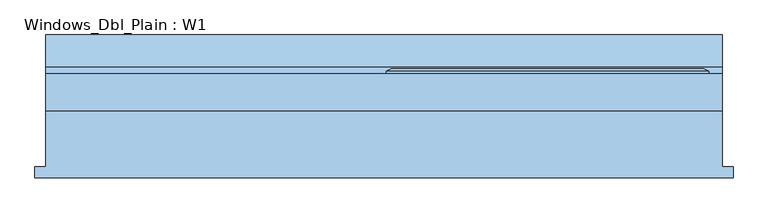
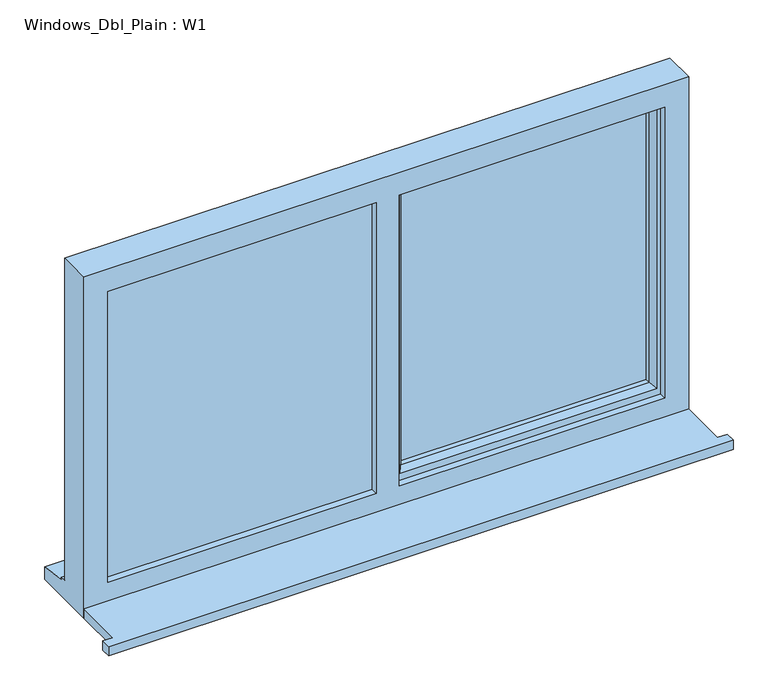
"""IFC4 building model written with IfcOpenShell, lengths in millimetres: window geometry, Windows_Dbl_Plain : W1."""

from ifc_helpers import new_model, si_unit, frame, origin, place, context, project, spatial, polyline, outline, extrude, faceted_brep, source, transform, mapped, element, save


def windows_dbl_plain_w1_b9c38b89(model_context):
    return source(origin(), model_context, "Body", "SolidModel", [
        extrude(outline(polyline([(-1072.0, -146.0834322), (-1072.0, -121.0834322), (-1047.0, -121.0834322), (-1047.0, 4.9965678), (477.0, 4.9965678), (477.0, -121.0834322), (502.0, -121.0834322), (502.0, -146.0834322), (-1072.0, -146.0834322)])), frame((0.0, 0.0, 1200.0), z_axis=(0.0, 0.0, 1.0), x_axis=(1.0, 0.0, 0.0)), (0.0, 0.0, 1.0), 25.0),
        faceted_brep([(-280.0, 87.9965678, 2080.0), (-280.0, 93.7700705, 2080.0), (-280.0, 93.7700705, 1253.0), (-280.0, 87.9965678, 1253.0), (-270.0, 22.9965678, 2070.0), (-270.0, 87.9965678, 2070.0), (-270.0, 87.9965678, 1263.0), (-270.0, 22.9965678, 1263.0), (-230.0, 37.4894677, 2030.0), (-240.1480377, 22.9965678, 2040.1480377), (-240.1480377, 22.9965678, 1292.8519623), (-230.0, 37.4894677, 1303.0), (-230.0, 51.9965678, 2030.0), (-230.0, 51.9965678, 1303.0), (-240.0, 75.9965678, 2040.0), (-240.0, 51.9965678, 2040.0), (-240.0, 51.9965678, 1293.0), (-240.0, 75.9965678, 1293.0), (-230.0, 93.7700705, 2030.0), (-230.0, 75.9965678, 2030.0), (-230.0, 75.9965678, 1303.0), (-230.0, 93.7700705, 1303.0), (-247.4457548, 99.5435732, 2047.4457548), (-247.4457548, 99.5435732, 1285.5542452), (-269.2153903, 99.5435732, 2069.2153903), (-269.2153903, 99.5435732, 1263.7846097), (447.0, 93.7700705, 1253.0), (447.0, 87.9965678, 1253.0), (437.0, 87.9965678, 1263.0), (437.0, 22.9965678, 1263.0), (407.1480377, 22.9965678, 1292.8519623), (397.0, 37.4894677, 1303.0), (397.0, 51.9965678, 1303.0), (407.0, 51.9965678, 1293.0), (407.0, 75.9965678, 1293.0), (397.0, 75.9965678, 1303.0), (397.0, 93.7700705, 1303.0), (414.4457548, 99.5435732, 1285.5542452), (436.2153903, 99.5435732, 1263.7846097), (447.0, 93.7700705, 2080.0), (447.0, 87.9965678, 2080.0), (437.0, 87.9965678, 2070.0), (437.0, 22.9965678, 2070.0), (407.1480377, 22.9965678, 2040.1480377), (397.0, 37.4894677, 2030.0), (397.0, 51.9965678, 2030.0), (407.0, 51.9965678, 2040.0), (407.0, 75.9965678, 2040.0), (397.0, 75.9965678, 2030.0), (397.0, 93.7700705, 2030.0), (414.4457548, 99.5435732, 2047.4457548), (436.2153903, 99.5435732, 2069.2153903)], [[[0, 1, 2, 3]], [[4, 5, 6, 7]], [[8, 9, 10, 11]], [[12, 8, 11, 13]], [[14, 15, 16, 17]], [[18, 19, 20, 21]], [[22, 18, 21, 23]], [[1, 24, 25, 2]], [[3, 2, 26, 27]], [[7, 6, 28, 29]], [[11, 10, 30, 31]], [[13, 11, 31, 32]], [[17, 16, 33, 34]], [[21, 20, 35, 36]], [[23, 21, 36, 37]], [[2, 25, 38, 26]], [[27, 26, 39, 40]], [[29, 28, 41, 42]], [[31, 30, 43, 44]], [[32, 31, 44, 45]], [[34, 33, 46, 47]], [[36, 35, 48, 49]], [[37, 36, 49, 50]], [[26, 38, 51, 39]], [[40, 39, 1, 0]], [[3, 27, 40, 0], [5, 41, 28, 6]], [[42, 41, 5, 4]], [[7, 29, 42, 4], [9, 43, 30, 10]], [[44, 43, 9, 8]], [[45, 44, 8, 12]], [[15, 46, 33, 16], [13, 32, 45, 12]], [[47, 46, 15, 14]], [[17, 34, 47, 14], [19, 48, 35, 20]], [[49, 48, 19, 18]], [[50, 49, 18, 22]], [[24, 51, 38, 25], [23, 37, 50, 22]], [[39, 51, 24, 1]]]),
        extrude(outline(polyline([(2050.0, -310.0), (2070.0, -310.0), (2070.0, -1007.0), (1263.0, -1007.0), (1263.0, -310.0), (1283.0, -310.0), (1283.0, -987.0), (2050.0, -987.0), (2050.0, -310.0)])), frame((0.0, 46.9965678, 0.0), z_axis=(0.0, 1.0, 0.0), x_axis=(0.0, 0.0, 1.0)), (0.0, 0.0, 1.0), 41.0),
        faceted_brep([(477.0, 4.9965678, 2110.0), (-1047.0, 4.9965678, 2110.0), (-1047.0, 4.9965678, 1200.0), (477.0, 4.9965678, 1200.0), (417.0, 4.9965678, 2050.0), (417.0, 4.9965678, 1275.0), (-252.0, 4.9965678, 1275.0), (-252.0, 4.9965678, 2050.0), (-310.0, 4.9965678, 2050.0), (-310.0, 4.9965678, 1275.0), (-987.0, 4.9965678, 1275.0), (-987.0, 4.9965678, 2050.0), (-1047.0, 87.9965678, 2110.0), (-1047.0, 87.9965678, 1251.0), (-1047.0, 102.9965678, 1249.68767), (-1047.0, 102.9965678, 1244.7449676), (-1047.0, 175.4965678, 1233.8088847), (-1047.0, 175.4965678, 1200.0), (477.0, 87.9965678, 2110.0), (477.0, 87.9965678, 1251.0), (-1007.0, 87.9965678, 2070.0), (-1007.0, 87.9965678, 1263.0), (-310.0, 87.9965678, 1263.0), (-310.0, 87.9965678, 2070.0), (-270.0, 87.9965678, 2070.0), (-270.0, 87.9965678, 1263.0), (437.0, 87.9965678, 1263.0), (437.0, 87.9965678, 2070.0), (-1007.0, 22.9965678, 2070.0), (-1007.0, 22.9965678, 1263.0), (-300.0, 22.9965678, 2070.0), (-300.0, 22.9965678, 1263.0), (-310.0, 22.9965678, 2050.0), (-987.0, 22.9965678, 2050.0), (-987.0, 22.9965678, 1275.0), (-310.0, 22.9965678, 1275.0), (-270.0, 22.9965678, 2070.0), (437.0, 22.9965678, 2070.0), (437.0, 22.9965678, 1263.0), (-270.0, 22.9965678, 1263.0), (417.0, 22.9965678, 2050.0), (-252.0, 22.9965678, 2050.0), (-252.0, 22.9965678, 1275.0), (417.0, 22.9965678, 1275.0), (-310.0, 46.9965678, 2070.0), (-300.0, 46.9965678, 2070.0), (477.0, 175.4965678, 1200.0), (477.0, 175.4965678, 1233.8088847), (477.0, 102.9965678, 1244.7449676), (477.0, 102.9965678, 1249.68767), (-300.0, 46.9965678, 1263.0), (-310.0, 46.9965678, 1263.0)], [[[0, 1, 2, 3], [4, 5, 6, 7], [8, 9, 10, 11]], [[2, 1, 12, 13, 14, 15, 16, 17]], [[13, 12, 18, 19], [20, 21, 22, 23], [24, 25, 26, 27]], [[21, 20, 28, 29]], [[28, 30, 31, 29], [32, 33, 34, 35]], [[36, 37, 38, 39], [40, 41, 42, 43]], [[33, 11, 10, 34]], [[1, 0, 18, 12]], [[28, 20, 23, 44, 45, 30]], [[27, 37, 36, 24]], [[11, 33, 32, 8]], [[40, 4, 7, 41]], [[19, 18, 0, 3, 46, 47, 48, 49]], [[27, 26, 38, 37]], [[4, 40, 43, 5]], [[45, 50, 31, 30]], [[50, 45, 44, 51]], [[51, 44, 23, 22]], [[25, 24, 36, 39]], [[41, 7, 6, 42]], [[8, 32, 35, 9]], [[46, 3, 2, 17]], [[47, 46, 17, 16]], [[48, 47, 16, 15]], [[49, 48, 15, 14]], [[19, 49, 14, 13]], [[22, 21, 29, 31, 50, 51]], [[26, 25, 39, 38]], [[6, 5, 43, 42]], [[35, 34, 10, 9]]]),
        extrude(outline(polyline([(-1007.0, 46.9965678), (-300.0, 46.9965678), (-300.0, 22.9965678), (-1007.0, 22.9965678), (-1007.0, 46.9965678)])), frame((0.0, 0.0, 1263.0), z_axis=(0.0, 0.0, 1.0), x_axis=(1.0, 0.0, 0.0)), (0.0, 0.0, 1.0), 807.0),
        extrude(outline(polyline([(407.0, 51.9965678), (-240.0, 51.9965678), (-240.0, 75.9965678), (407.0, 75.9965678), (407.0, 51.9965678)])), frame((0.0, 0.0, 1293.0), z_axis=(0.0, 0.0, 1.0), x_axis=(1.0, 0.0, 0.0)), (0.0, 0.0, 1.0), 747.0),
    ])


if __name__ == "__main__":
    model = new_model("IFC4")
    model_context = context("Model", 3, world=origin())
    ifc_project = project(units=[si_unit("LENGTHUNIT", "METRE", prefix="MILLI")], contexts=[model_context])
    site = spatial("IfcSite", under=ifc_project)
    building = spatial("IfcBuilding", under=site)
    placement = place(None, origin())
    windows_dbl_plain_w1_shape = windows_dbl_plain_w1_b9c38b89(model_context)
    element("IfcWindow", 1, ObjectType="Windows_Dbl_Plain : W1", at=placement, inside=building, context=model_context, shape_type="MappedRepresentation", body=[
        mapped(windows_dbl_plain_w1_shape, transform((0.0, 0.0, 0.0), x_axis=(1.0, 0.0, 0.0), y_axis=(0.0, 1.0, 0.0), z_axis=(0.0, 0.0, 1.0))),
    ])
    save(model, "model.ifc")

# Revit data of these elements
# Type "Windows_Dbl_Plain : W1"
#   Type Mark = "56"
#   Operation = "DoublePanelVertical"
#   Construction Type Id = "GSP4R"
#   Manufacturer = "Revit"
#   Keynote = "L10"
#   Analytic Construction = "1/8 in Pilkington single glazing"
#   Wrap Layers (Ext) from Ext = 0.336286 ft
#   Wrap Layers (Int) from Ext = 0.582349 ft
#   Window Board Projection = 0.082021 ft
#   Window Board Extension = 0.082021 ft
#   Visual Light Transmittance = 0.9
#   Solar Heat Gain Coefficient = 0.78
#   Rough Width = 5.0 ft
#   Rough Height = 2.985564 ft
#   Height = 2.985564 ft
#   Width = 5.0 ft
#   Heat Transfer Coefficient (U) = 3.6886 W/(m²·K)
#   Glazing Thickness = 0.07874 ft
#   FrameOffset - External = 0.164042 ft
#   Frame Depth = 0.213255 ft
#   Default Head Height = 6.922572 ft
#   Cill Depth = 0.287073 ft
#   Cavity Closer Width = 0.164042 ft
#   Cavity Closer Offset from Ext = 0.336286 ft
#   Cavity Closer Depth = 0.278871 ft
#   Vis - Cavity Closers = yes
#   Define Thermal Properties by = 1
#   Material Trim = Window Frame
#   Material Glass = Glass
#   Material Frame = Window Frame
#   Wall Closure = (empty or 0)
# Element 1 (IfcWindow, "Windows_Dbl_Plain : W1")
#   Materials on its faces: "Window Frame", "Glass"
# Materials
#   "Window Frame": colour RGB 249 249 249, transparency 0, Keynote = "L10", Cost = 0
#   "Glass": class "Glass", colour RGB 0 128 192, transparency 0.9, Description = "Soda Lime Glass", Cost = 0
